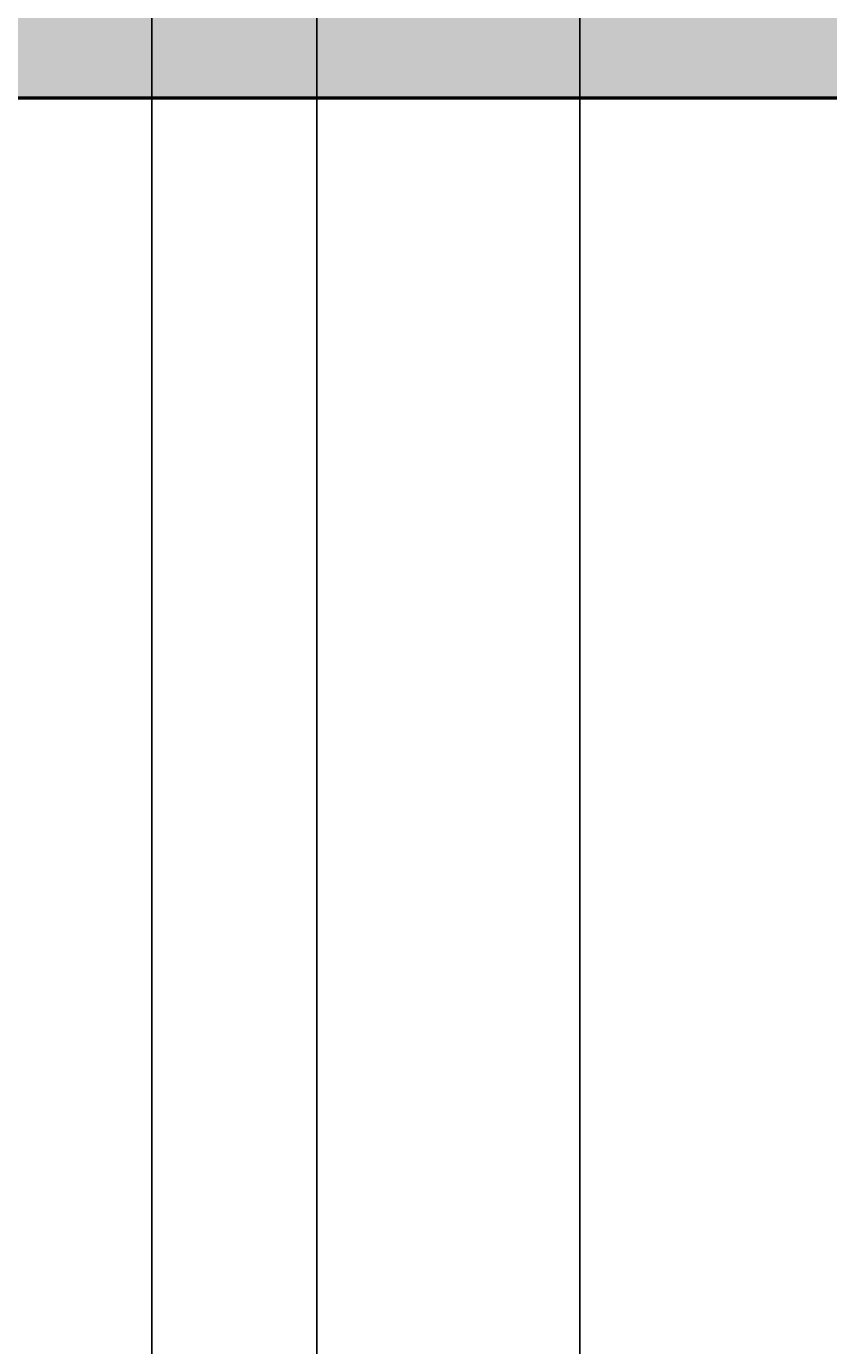
# Model space of a CAD drawing. Units: inches. Extents: x 2231 to 2461, y 2045 to 2455.
# Tile 64 of 95: x 2393 to 2416, y 2296 to 2333. Entities that reach past the tile are written whole.
import ezdxf

# ---------------------------------------------------------------- set-up
doc = ezdxf.new("R2010")
doc.units = ezdxf.units.IN
doc.layers.add('A-ANNO-DIMS', color=2, linetype='Continuous', lineweight=18)
doc.layers.add('A-WALL', color=7, linetype='Continuous', lineweight=50)
doc.layers.add('A-WALL-PATT', color=18, linetype='Continuous', lineweight=13, true_color=0x000000)
doc.styles.get("Standard").update_dxf_attribs({"font": 'arial.ttf'})
doc.dimstyles.get("Standard").update_dxf_attribs({"dimtxt": 0.18, "dimasz": 0.18, "dimexe": 0.18, "dimexo": 0.0625, "dimgap": 0.09, "dimtad": 0, "dimtih": 1, "dimtoh": 1, "dimdec": 4, "dimzin": 0, "dimdsep": 46, "dimtxsty": 'Standard', "dimcen": 0.09, "dimadec": 0, "dimazin": 0, "dimtfac": 1, "dimtdec": 4, "dimtofl": 0, "dimtmove": 0, "dimatfit": 3, "dimfxl": 1, "dimtolj": 1, "dimtzin": 0, "dimarcsym": 0})

# ---------------------------------------------------------------- blocks, each defined once
blk = doc.blocks.new('*D42')
at = {"layer": 'A-ANNO-DIMS', "color": 0, "lineweight": -2, "transparency": 16777216}
for p, q in [((2396.794, 2286.895), (2396.794, 2454.645)), ((2432.794, 2286.895), (2432.794, 2454.645)), ((2396.974, 2454.465), (2414.575, 2454.465)), ((2432.614, 2454.465), (2415.012, 2454.465))]:
    blk.add_line(p, q, dxfattribs=at)
at = {"layer": 'A-ANNO-DIMS', "color": 0, "transparency": 16777216}
for points in [[(2396.974, 2454.495), (2396.974, 2454.435), (2396.794, 2454.465)], [(2432.614, 2454.495), (2432.614, 2454.435), (2432.794, 2454.465)]]:
    blk.add_solid(points, dxfattribs=at)
at = {"layer": 'Defpoints', "color": 0, "transparency": 16777216}
for p in [(2432.794, 2454.465), (2396.794, 2286.833), (2432.794, 2286.833)]:
    blk.add_point(p, dxfattribs=at)
at = {"layer": 'A-ANNO-DIMS', "color": 0, "transparency": 16777216, "insert": (2414.794, 2454.465), "char_height": 0.18, "attachment_point": 5}
blk.add_mtext('\\A1;36', dxfattribs=at)
blk = doc.blocks.new('*D59')
at = {"layer": 'A-ANNO-DIMS', "color": 0, "lineweight": -2, "transparency": 16777216}
for p, q in [((2408.794, 2182.895), (2408.794, 2454.645)), ((2432.794, 2182.895), (2432.794, 2454.645)), ((2408.974, 2454.465), (2420.573, 2454.465)), ((2432.614, 2454.465), (2421.014, 2454.465))]:
    blk.add_line(p, q, dxfattribs=at)
at = {"layer": 'A-ANNO-DIMS', "color": 0, "transparency": 16777216}
for points in [[(2408.974, 2454.495), (2408.974, 2454.435), (2408.794, 2454.465)], [(2432.614, 2454.495), (2432.614, 2454.435), (2432.794, 2454.465)]]:
    blk.add_solid(points, dxfattribs=at)
at = {"layer": 'Defpoints', "color": 0, "transparency": 16777216}
for p in [(2432.794, 2454.465), (2408.794, 2182.833), (2432.794, 2182.833)]:
    blk.add_point(p, dxfattribs=at)
at = {"layer": 'A-ANNO-DIMS', "color": 0, "transparency": 16777216, "insert": (2420.794, 2454.465), "char_height": 0.18, "attachment_point": 5}
blk.add_mtext('\\A1;24', dxfattribs=at)
blk = doc.blocks.new('*D66')
at = {"layer": 'A-ANNO-DIMS', "color": 0, "lineweight": -2, "transparency": 16777216}
for p, q in [((2348.189, 2096.895), (2348.189, 2454.645)), ((2408.794, 2096.895), (2408.794, 2454.645)), ((2348.369, 2454.465), (2378.167, 2454.465)), ((2408.614, 2454.465), (2378.815, 2454.465))]:
    blk.add_line(p, q, dxfattribs=at)
at = {"layer": 'A-ANNO-DIMS', "color": 0, "transparency": 16777216}
for points in [[(2348.369, 2454.495), (2348.369, 2454.435), (2348.189, 2454.465)], [(2408.614, 2454.495), (2408.614, 2454.435), (2408.794, 2454.465)]]:
    blk.add_solid(points, dxfattribs=at)
at = {"layer": 'Defpoints', "color": 0, "transparency": 16777216}
for p in [(2408.794, 2454.465), (2348.189, 2096.833), (2408.794, 2096.833)]:
    blk.add_point(p, dxfattribs=at)
at = {"layer": 'A-ANNO-DIMS', "color": 0, "transparency": 16777216, "insert": (2378.491, 2454.465), "char_height": 0.18, "attachment_point": 5}
blk.add_mtext('\\A1;60.6', dxfattribs=at)
blk = doc.blocks.new('*D71')
at = {"layer": 'A-ANNO-DIMS', "color": 0, "lineweight": -2, "transparency": 16777216}
for p, q in [((2401.422, 2092.979), (2401.422, 2454.645)), ((2408.794, 2096.895), (2408.794, 2454.645)), ((2401.602, 2454.465), (2404.732, 2454.465)), ((2408.614, 2454.465), (2405.483, 2454.465))]:
    blk.add_line(p, q, dxfattribs=at)
at = {"layer": 'A-ANNO-DIMS', "color": 0, "transparency": 16777216}
for points in [[(2401.602, 2454.495), (2401.602, 2454.435), (2401.422, 2454.465)], [(2408.614, 2454.495), (2408.614, 2454.435), (2408.794, 2454.465)]]:
    blk.add_solid(points, dxfattribs=at)
at = {"layer": 'Defpoints', "color": 0, "transparency": 16777216}
for p in [(2408.794, 2454.465), (2408.794, 2096.833), (2401.422, 2092.917)]:
    blk.add_point(p, dxfattribs=at)
at = {"layer": 'A-ANNO-DIMS', "color": 0, "transparency": 16777216, "insert": (2405.108, 2454.465), "char_height": 0.18, "attachment_point": 5}
blk.add_mtext('\\A1;7.371', dxfattribs=at)
blk = doc.blocks.new('*D72')
at = {"layer": 'A-ANNO-DIMS', "color": 0, "lineweight": -2, "transparency": 16777216}
for p, q in [((2384.543, 2145.12), (2384.543, 2454.645)), ((2408.794, 2150.677), (2408.794, 2454.645)), ((2384.723, 2454.465), (2396.272, 2454.465)), ((2408.614, 2454.465), (2397.064, 2454.465))]:
    blk.add_line(p, q, dxfattribs=at)
at = {"layer": 'A-ANNO-DIMS', "color": 0, "transparency": 16777216}
for points in [[(2384.723, 2454.495), (2384.723, 2454.435), (2384.543, 2454.465)], [(2408.614, 2454.495), (2408.614, 2454.435), (2408.794, 2454.465)]]:
    blk.add_solid(points, dxfattribs=at)
at = {"layer": 'Defpoints', "color": 0, "transparency": 16777216}
for p in [(2408.794, 2454.465), (2408.794, 2150.615), (2384.543, 2145.058)]:
    blk.add_point(p, dxfattribs=at)
at = {"layer": 'A-ANNO-DIMS', "color": 0, "transparency": 16777216, "insert": (2396.668, 2454.465), "char_height": 0.18, "attachment_point": 5}
blk.add_mtext('\\A1;24.25', dxfattribs=at)

msp = doc.modelspace()

# ---------------------------------------------------------------- hatches: boundary and pattern name
at = {"layer": 'A-WALL-PATT'}
h = msp.add_hatch(color=256, dxfattribs=at)
h.dxf.hatch_style = 1
h.paths.add_polyline_path([(2441.7935, 2269.1535), (2432.7935, 2269.1535), (2432.7935, 2186.8328), (2396.7935, 2186.8328), (2396.7935, 2286.8328), (2394.7935, 2286.8328), (2394.7935, 2186.8328), (2334.7935, 2186.8328), (2334.7935, 2182.8328), (2432.7935, 2182.8328), (2432.7935, 2072.8328), (2416.6639, 2072.8328), (2416.6639, 2063.8328), (2441.7935, 2063.8328)])
h.paths.add_polyline_path([(2368.6639, 2072.8328), (2367.04, 2072.8328), (2330.7942, 2072.8328), (2330.7397, 2063.8328), (2368.6639, 2063.8328)])
h.paths.add_polyline_path([(2300.7392, 2068.3328), (2300.7392, 2072.8328), (2298.7935, 2072.8328), (2294.7935, 2072.8328), (2258.7935, 2072.8328), (2258.7935, 2120.8328), (2294.7935, 2120.8328), (2298.7935, 2120.8328), (2298.7935, 2128.8328), (2294.7935, 2128.8328), (2294.7935, 2124.8328), (2258.7935, 2124.8328), (2258.7935, 2182.8328), (2294.7935, 2182.8328), (2294.7935, 2174.8328), (2298.7935, 2174.8328), (2298.7935, 2182.8328), (2304.7935, 2182.8328), (2304.7935, 2186.8328), (2258.7935, 2186.8328), (2258.7935, 2221.999), (2249.7935, 2221.999), (2249.7935, 2063.8328), (2300.7392, 2063.8328)])
h.paths.add_polyline_path([(2391.9338, 2435.8328), (2333.82, 2435.8328), (2333.82, 2426.8328), (2368.7935, 2426.8328), (2368.7935, 2374.9508), (2368.7935, 2370.8328), (2372.3935, 2370.8328), (2372.7935, 2370.8328), (2372.7935, 2426.8328), (2391.9338, 2426.8328)])
h.paths.add_polyline_path([(2441.7935, 2435.8328), (2415.9338, 2435.8328), (2415.9338, 2426.8328), (2432.7935, 2426.8328), (2432.7935, 2334.8328), (2372.7935, 2334.8328), (2372.7935, 2346.8328), (2368.7935, 2346.8328), (2368.7935, 2306.8328), (2360.7935, 2306.8328), (2360.7935, 2302.8328), (2368.7935, 2302.8328), (2372.7935, 2302.8328), (2372.7935, 2330.8328), (2432.7935, 2330.8328), (2432.7935, 2317.1535), (2441.7935, 2317.1535)])
h.paths.add_polyline_path([(2285.82, 2435.8328), (2249.7935, 2435.8328), (2249.7935, 2269.999), (2258.7935, 2269.999), (2258.7935, 2302.8328), (2318.8168, 2302.8328), (2330.7935, 2302.8328), (2330.7935, 2306.8328), (2258.7935, 2306.8328), (2258.7935, 2426.8328), (2285.82, 2426.8328)])

# ---------------------------------------------------------------- linework, layer by layer
at = {"layer": 'A-WALL'}
msp.add_line((2372.7935, 2330.8328), (2432.7935, 2330.8328), dxfattribs=at)

# ---------------------------------------------------------------- dimensions: what is measured, and where the dimension line sits
at = {"layer": 'A-ANNO-DIMS'}
for base, p1, p2, override, picture, middle in [((2408.7935, 2454.4653), (2348.1888, 2096.8328), (2408.7935, 2096.8328), {"dimdec": 1, "dimlfac": 1, "dimrnd": 0, "dimzin": 0, "dimdsep": 46, "dimlunit": 2}, '*D66', (2378.4912, 2454.4653)), ((2408.7935, 2454.4653), (2384.5428, 2145.0576), (2408.7935, 2150.6145), {"dimdec": 2, "dimlfac": 1, "dimrnd": 0, "dimzin": 0, "dimdsep": 46, "dimlunit": 2}, '*D72', (2396.6682, 2454.4653)), ((2432.7935, 2454.4653), (2396.7935, 2286.8328), (2432.7935, 2286.8328), {"dimdec": 0, "dimlfac": 1, "dimrnd": 0, "dimzin": 0, "dimdsep": 46, "dimlunit": 2}, '*D42', (2414.7935, 2454.4653)), ((2408.7935, 2454.4653), (2401.4221, 2092.9167), (2408.7935, 2096.8328), {"dimdec": 3, "dimlfac": 1, "dimrnd": 0, "dimzin": 0, "dimdsep": 46, "dimlunit": 2}, '*D71', (2405.1078, 2454.4653)), ((2432.7935, 2454.4653), (2408.7935, 2182.8328), (2432.7935, 2182.8328), {"dimdec": 0, "dimlfac": 1, "dimrnd": 0, "dimzin": 0, "dimdsep": 46, "dimlunit": 2}, '*D59', (2420.7935, 2454.4653))]:
    dim = msp.add_linear_dim(base=base, p1=p1, p2=p2, dimstyle='Standard', override=override, dxfattribs=at)
    dim.commit()
    dim.dimension.update_dxf_attribs({"geometry": picture, "text_midpoint": middle})

doc.saveas('drawing.dxf')
